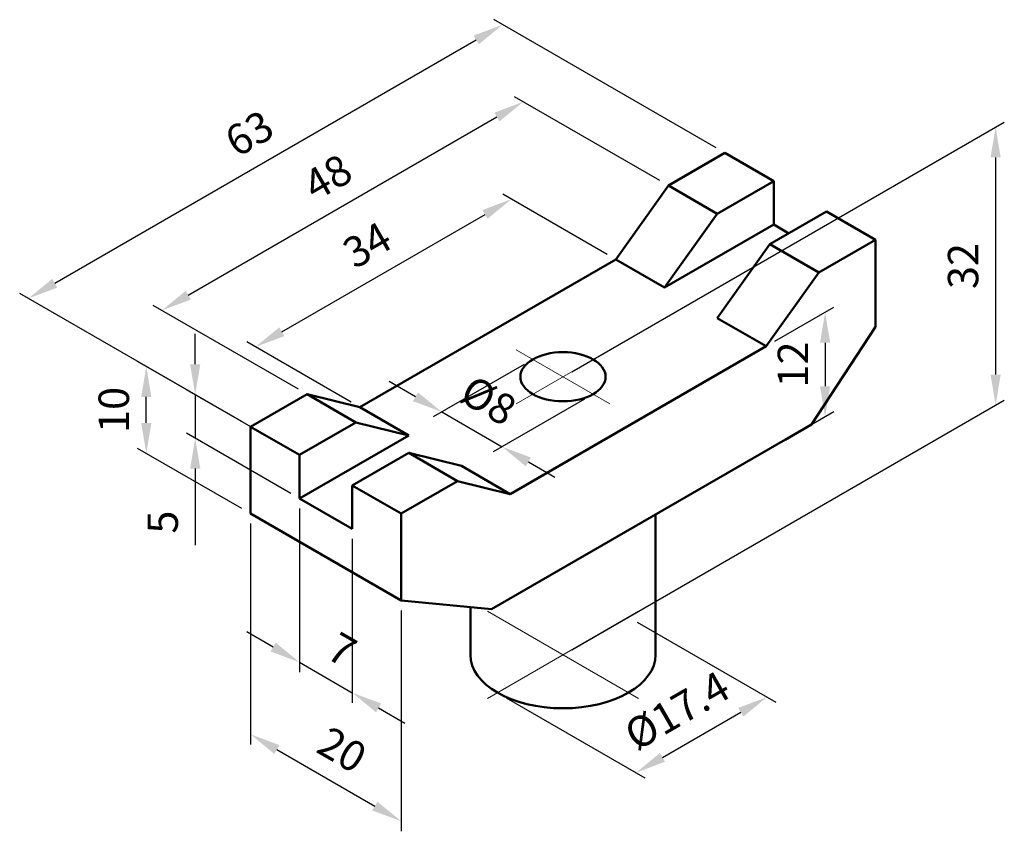
# Model space of a CAD drawing. Units: millimetres. Extents: x 2104 to 2217, y 1234 to 1327.
import ezdxf

# ---------------------------------------------------------------- set-up
doc = ezdxf.new("R2010")
doc.units = ezdxf.units.MM
doc.linetypes.add('CENTER', pattern=[50.8, 31.75, -6.35, 6.35, -6.35])
for name, color, linetype, lineweight in [('M-CNTR', 4, 'CENTER', 18), ('M-DIMS', 3, 'Continuous', 25), ('M-OUTL', 7, 'Continuous', 50)]:
    doc.layers.add(name, color=color, linetype=linetype, lineweight=lineweight)
doc.styles.get("Standard").update_dxf_attribs({"font": 'arial.ttf'})
doc.dimstyles.new('AM_ISO$0', dxfattribs={"dimtxt": 3.5, "dimasz": 3.5, "dimexe": 1, "dimexo": 1, "dimgap": 1.5, "dimtad": 1, "dimdsep": 46, "dimtxsty": 'Standard', "dimcen": 0, "dimclrd": 256, "dimclre": 256, "dimclrt": 2, "dimadec": 0, "dimazin": 2, "dimtp": 0.1, "dimtm": 0.1, "dimtfac": 0.71, "dimtdec": 3, "dimtmove": 0, "dimatfit": 3, "dimfxl": 1, "dimlwd": -1, "dimlwe": -1, "dimarcsym": 1})

# ---------------------------------------------------------------- blocks, each defined once
blk = doc.blocks.new('*D3')
at = {"layer": 'Defpoints', "color": 0, "transparency": 16777216}
for p in [(2159.14, 1326.8), (2184.7, 1312.04), (2130.15, 1280.54)]:
    blk.add_point(p, dxfattribs=at)
at = {"layer": 'M-DIMS', "color": 0, "linetype": 'ByBlock', "transparency": 16777216}
for p, q in [((2183.7, 1312.62), (2158.14, 1327.38)), ((2107.61, 1297.05), (2156.11, 1325.05)), ((2129.15, 1281.12), (2103.58, 1295.88))]:
    blk.add_line(p, q, dxfattribs=at)
at = {"layer": 'M-DIMS', "color": 0, "transparency": 16777216}
for points in [[(2155.82, 1325.55), (2156.4, 1324.54), (2159.14, 1326.8)], [(2107.32, 1297.55), (2107.9, 1296.54), (2104.58, 1295.3)]]:
    blk.add_solid(points, dxfattribs=at)
at = {"layer": 'M-DIMS', "color": 0, "transparency": 16777216, "insert": (2130.22, 1313.9), "char_height": 3.5, "attachment_point": 5, "rotation": 30}
blk.add_mtext('63', dxfattribs=at)
blk = doc.blocks.new('*D4')
at = {"layer": 'Defpoints', "color": 0, "transparency": 16777216}
for p in [(2161.52, 1317.93), (2178.21, 1308.29), (2136.64, 1284.29)]:
    blk.add_point(p, dxfattribs=at)
at = {"layer": 'M-DIMS', "color": 0, "linetype": 'ByBlock', "transparency": 16777216}
for p, q in [((2177.21, 1308.87), (2160.52, 1318.5)), ((2122.98, 1295.68), (2158.49, 1316.18)), ((2135.64, 1284.87), (2118.95, 1294.5))]:
    blk.add_line(p, q, dxfattribs=at)
at = {"layer": 'M-DIMS', "color": 0, "transparency": 16777216}
for points in [[(2158.2, 1316.68), (2158.78, 1315.67), (2161.52, 1317.93)], [(2122.69, 1296.18), (2123.27, 1295.17), (2119.95, 1293.93)]]:
    blk.add_solid(points, dxfattribs=at)
at = {"layer": 'M-DIMS', "color": 0, "transparency": 16777216, "insert": (2139.24, 1308.86), "char_height": 3.5, "attachment_point": 5, "rotation": 30}
blk.add_mtext('48', dxfattribs=at)
blk = doc.blocks.new('*D5')
at = {"layer": 'Defpoints', "color": 0, "transparency": 16777216}
for p in [(2160.15, 1306.72), (2172.15, 1299.79), (2142.7, 1282.79)]:
    blk.add_point(p, dxfattribs=at)
at = {"layer": 'M-DIMS', "color": 0, "linetype": 'ByBlock', "transparency": 16777216}
for p, q in [((2171.15, 1300.37), (2159.15, 1307.3)), ((2133.73, 1291.47), (2157.12, 1304.97)), ((2141.7, 1283.37), (2129.7, 1290.3))]:
    blk.add_line(p, q, dxfattribs=at)
at = {"layer": 'M-DIMS', "color": 0, "transparency": 16777216}
for points in [[(2156.82, 1305.47), (2157.41, 1304.46), (2160.15, 1306.72)], [(2133.44, 1291.97), (2134.03, 1290.96), (2130.7, 1289.72)]]:
    blk.add_solid(points, dxfattribs=at)
at = {"layer": 'M-DIMS', "color": 0, "transparency": 16777216, "insert": (2143.78, 1301.07), "char_height": 3.5, "attachment_point": 5, "rotation": 30}
blk.add_mtext('34', dxfattribs=at)
blk = doc.blocks.new('*D6')
at = {"layer": 'Defpoints', "color": 0, "transparency": 16777216}
for p in [(2118.15, 1287.47), (2130.15, 1280.54), (2130.15, 1270.54)]:
    blk.add_point(p, dxfattribs=at)
at = {"layer": 'M-DIMS', "color": 0, "linetype": 'ByBlock', "transparency": 16777216}
for p, q in [((2129.15, 1281.12), (2117.15, 1288.05)), ((2118.15, 1280.97), (2118.15, 1283.97)), ((2129.15, 1271.12), (2117.15, 1278.05))]:
    blk.add_line(p, q, dxfattribs=at)
at = {"layer": 'M-DIMS', "color": 0, "transparency": 16777216}
for points in [[(2117.56, 1283.97), (2118.73, 1283.97), (2118.15, 1287.47)], [(2117.56, 1280.97), (2118.73, 1280.97), (2118.15, 1277.47)]]:
    blk.add_solid(points, dxfattribs=at)
at = {"layer": 'M-DIMS', "color": 0, "transparency": 16777216, "insert": (2114.86, 1282.47), "char_height": 3.5, "attachment_point": 5, "rotation": 90}
blk.add_mtext('10', dxfattribs=at)
blk = doc.blocks.new('*D7')
at = {"layer": 'Defpoints', "color": 0, "transparency": 16777216}
for p in [(2135.77, 1272.29), (2141.84, 1268.79), (2141.84, 1249.93)]:
    blk.add_point(p, dxfattribs=at)
at = {"layer": 'M-DIMS', "color": 0, "linetype": 'ByBlock', "transparency": 16777216}
for p, q in [((2135.77, 1271.14), (2135.77, 1252.28)), ((2141.84, 1267.64), (2141.84, 1248.78)), ((2132.74, 1255.18), (2129.71, 1256.93)), ((2135.77, 1253.43), (2141.84, 1249.93)), ((2144.87, 1248.18), (2147.9, 1246.43))]:
    blk.add_line(p, q, dxfattribs=at)
at = {"layer": 'M-DIMS', "color": 0, "transparency": 16777216}
for points in [[(2133.03, 1255.69), (2132.45, 1254.68), (2135.77, 1253.43)], [(2145.16, 1248.69), (2144.58, 1247.68), (2141.84, 1249.93)]]:
    blk.add_solid(points, dxfattribs=at)
at = {"layer": 'M-DIMS', "color": 0, "transparency": 16777216, "insert": (2140.43, 1254.5), "char_height": 3.5, "attachment_point": 5, "rotation": 330}
blk.add_mtext('7', dxfattribs=at)
blk = doc.blocks.new('*D8')
at = {"layer": 'Defpoints', "color": 0, "transparency": 16777216}
for p in [(2130.15, 1270.54), (2147.47, 1260.54), (2147.47, 1235.14)]:
    blk.add_point(p, dxfattribs=at)
at = {"layer": 'M-DIMS', "color": 0, "linetype": 'ByBlock', "transparency": 16777216}
for p, q in [((2130.15, 1269.39), (2130.15, 1243.98)), ((2147.47, 1259.39), (2147.47, 1233.98)), ((2133.18, 1243.39), (2144.43, 1236.89))]:
    blk.add_line(p, q, dxfattribs=at)
at = {"layer": 'M-DIMS', "color": 0, "transparency": 16777216}
for points in [[(2133.47, 1243.89), (2132.88, 1242.88), (2130.15, 1245.14)], [(2144.73, 1237.39), (2144.14, 1236.38), (2147.47, 1235.14)]]:
    blk.add_solid(points, dxfattribs=at)
at = {"layer": 'M-DIMS', "color": 0, "transparency": 16777216, "insert": (2140.45, 1242.98), "char_height": 3.5, "attachment_point": 5, "rotation": 330}
blk.add_mtext('20', dxfattribs=at)
blk = doc.blocks.new('*D9')
at = {"layer": 'Defpoints', "color": 0, "transparency": 16777216}
for p in [(2162.62, 1288.29), (2169.55, 1284.29), (2159.07, 1278.24)]:
    blk.add_point(p, dxfattribs=at)
at = {"layer": 'M-DIMS', "color": 0, "linetype": 'ByBlock', "transparency": 16777216}
for p, q in [((2161.62, 1287.71), (2151.14, 1281.66)), ((2149.11, 1283.99), (2146.08, 1285.74)), ((2168.55, 1283.71), (2158.07, 1277.66)), ((2152.14, 1282.24), (2159.07, 1278.24)), ((2162.1, 1276.49), (2165.13, 1274.74))]:
    blk.add_line(p, q, dxfattribs=at)
at = {"layer": 'M-DIMS', "color": 0, "transparency": 16777216}
for points in [[(2149.4, 1284.49), (2148.82, 1283.48), (2152.14, 1282.24)], [(2162.39, 1276.99), (2161.81, 1275.98), (2159.07, 1278.24)]]:
    blk.add_solid(points, dxfattribs=at)
at = {"layer": 'M-DIMS', "color": 0, "transparency": 16777216, "insert": (2157.3, 1283.17), "char_height": 3.5, "attachment_point": 5, "rotation": 330}
blk.add_mtext('%%C8', dxfattribs=at)
blk = doc.blocks.new('*D10')
at = {"layer": 'Defpoints', "color": 0, "transparency": 16777216}
for p in [(2166.09, 1286.29), (2215.86, 1283.03), (2166.09, 1254.29)]:
    blk.add_point(p, dxfattribs=at)
at = {"layer": 'M-DIMS', "color": 0, "linetype": 'ByBlock', "transparency": 16777216}
for p, q in [((2167.09, 1286.87), (2216.86, 1315.6)), ((2215.86, 1311.53), (2215.86, 1286.53)), ((2167.09, 1254.87), (2216.86, 1283.6))]:
    blk.add_line(p, q, dxfattribs=at)
at = {"layer": 'M-DIMS', "color": 0, "transparency": 16777216}
for points in [[(2215.27, 1311.53), (2216.44, 1311.53), (2215.86, 1315.03)], [(2215.27, 1286.53), (2216.44, 1286.53), (2215.86, 1283.03)]]:
    blk.add_solid(points, dxfattribs=at)
at = {"layer": 'M-DIMS', "color": 0, "transparency": 16777216, "insert": (2212.57, 1299.03), "char_height": 3.5, "attachment_point": 5, "rotation": 90}
blk.add_mtext('32', dxfattribs=at)
blk = doc.blocks.new('*D11')
at = {"layer": 'Defpoints', "color": 0, "transparency": 16777216}
for p in [(2189.47, 1289.79), (2196.24, 1281.7), (2189.37, 1277.73)]:
    blk.add_point(p, dxfattribs=at)
at = {"layer": 'M-DIMS', "color": 0, "linetype": 'ByBlock', "transparency": 16777216}
for p, q in [((2190.47, 1290.37), (2197.24, 1294.28)), ((2196.24, 1290.2), (2196.24, 1285.2)), ((2190.37, 1278.31), (2197.24, 1282.28))]:
    blk.add_line(p, q, dxfattribs=at)
at = {"layer": 'M-DIMS', "color": 0, "transparency": 16777216}
for points in [[(2195.66, 1290.2), (2196.83, 1290.2), (2196.24, 1293.7)], [(2195.66, 1285.2), (2196.83, 1285.2), (2196.24, 1281.7)]]:
    blk.add_solid(points, dxfattribs=at)
at = {"layer": 'M-DIMS', "color": 0, "transparency": 16777216, "insert": (2192.99, 1287.7), "char_height": 3.5, "attachment_point": 5, "rotation": 90}
blk.add_mtext('12', dxfattribs=at)
blk = doc.blocks.new('*D12')
at = {"layer": 'Defpoints', "color": 0, "transparency": 16777216}
for p in [(2173.62, 1258.64), (2158.55, 1249.94), (2189.57, 1249.43)]:
    blk.add_point(p, dxfattribs=at)
at = {"layer": 'M-DIMS', "color": 0, "linetype": 'ByBlock', "transparency": 16777216}
for p, q in [((2174.62, 1258.06), (2190.57, 1248.85)), ((2159.55, 1249.36), (2175.5, 1240.15)), ((2177.53, 1242.48), (2186.54, 1247.68))]:
    blk.add_line(p, q, dxfattribs=at)
at = {"layer": 'M-DIMS', "color": 0, "transparency": 16777216}
for points in [[(2186.25, 1248.19), (2186.83, 1247.18), (2189.57, 1249.43)], [(2177.24, 1242.99), (2177.82, 1241.98), (2174.5, 1240.73)]]:
    blk.add_solid(points, dxfattribs=at)
at = {"layer": 'M-DIMS', "color": 0, "transparency": 16777216, "insert": (2179.43, 1247.48), "char_height": 3.5, "attachment_point": 5, "rotation": 30}
blk.add_mtext('%%C17.4', dxfattribs=at)
blk = doc.blocks.new('*D13')
at = {"layer": 'Defpoints', "color": 0, "transparency": 16777216}
for p in [(2123.77, 1279.22), (2135.77, 1277.29), (2135.77, 1272.29)]:
    blk.add_point(p, dxfattribs=at)
at = {"layer": 'M-DIMS', "color": 0, "linetype": 'ByBlock', "transparency": 16777216}
for p, q in [((2123.77, 1287.72), (2123.77, 1291.22)), ((2134.77, 1277.87), (2122.77, 1284.8)), ((2123.77, 1284.22), (2123.77, 1279.22)), ((2134.77, 1272.87), (2122.77, 1279.8)), ((2123.77, 1275.72), (2123.77, 1266.9))]:
    blk.add_line(p, q, dxfattribs=at)
at = {"layer": 'M-DIMS', "color": 0, "transparency": 16777216}
for points in [[(2123.19, 1287.72), (2124.36, 1287.72), (2123.77, 1284.22)], [(2123.19, 1275.72), (2124.36, 1275.72), (2123.77, 1279.22)]]:
    blk.add_solid(points, dxfattribs=at)
at = {"layer": 'M-DIMS', "color": 0, "transparency": 16777216, "insert": (2120.49, 1269.56), "char_height": 3.5, "attachment_point": 5, "rotation": 90}
blk.add_mtext('5', dxfattribs=at)

msp = doc.modelspace()

# ---------------------------------------------------------------- linework, layer by layer
at = {"layer": 'M-CNTR', "ltscale": 25}
for p, q in [((2160.701, 1289.398), (2171.469, 1283.181)), ((2160.701, 1283.181), (2171.469, 1289.398))]:
    msp.add_line(p, q, dxfattribs=at)
at = {"layer": 'M-CNTR'}
for p, q in [((2157.394, 1249.272), (2174.776, 1259.307)), ((2157.394, 1259.307), (2174.776, 1249.272))]:
    msp.add_line(p, q, dxfattribs=at)
at = {"layer": 'M-OUTL'}
for p, q in [((2184.705, 1312.04), (2178.209, 1308.29)), ((2184.705, 1312.04), (2190.334, 1308.79)), ((2183.839, 1305.04), (2190.334, 1308.79)), ((2190.334, 1308.79), (2190.334, 1303.79)), ((2178.209, 1308.29), (2172.147, 1299.79)), ((2183.839, 1305.04), (2178.209, 1308.29)), ((2183.839, 1305.04), (2177.776, 1296.54)), ((2189.901, 1301.54), (2196.396, 1305.29)), ((2196.396, 1305.29), (2202.025, 1302.04)), ((2190.334, 1303.79), (2177.776, 1296.54)), ((2190.334, 1303.79), (2192.066, 1302.79)), ((2189.901, 1301.54), (2183.839, 1293.04)), ((2195.53, 1298.29), (2189.901, 1301.54)), ((2202.025, 1302.04), (2195.53, 1298.29)), ((2202.025, 1302.04), (2195.53, 1298.29)), ((2202.025, 1292.04), (2202.025, 1302.04)), ((2202.025, 1302.04), (2202.025, 1297.04)), ((2202.025, 1302.04), (2202.025, 1292.04)), ((2142.702, 1282.79), (2172.147, 1299.79)), ((2177.776, 1296.54), (2172.147, 1299.79)), ((2195.53, 1298.29), (2189.468, 1289.79)), ((2189.468, 1289.79), (2183.839, 1293.04)), ((2194.664, 1280.79), (2202.025, 1292.04)), ((2189.468, 1289.79), (2160.023, 1272.79)), ((2130.145, 1280.54), (2136.64, 1284.29)), ((2136.64, 1284.29), (2130.145, 1280.54)), ((2136.64, 1284.29), (2142.269, 1281.04)), ((2136.64, 1284.29), (2142.702, 1282.79)), ((2148.332, 1279.54), (2142.702, 1282.79)), ((2130.145, 1270.54), (2130.145, 1280.54)), ((2130.145, 1280.54), (2135.774, 1277.29)), ((2130.145, 1280.54), (2130.145, 1275.54)), ((2135.774, 1277.29), (2142.269, 1281.04)), ((2135.774, 1277.29), (2142.269, 1281.04)), ((2142.269, 1281.04), (2148.332, 1279.54)), ((2157.858, 1259.54), (2194.664, 1280.79)), ((2194.664, 1280.79), (2191.633, 1279.04)), ((2191.633, 1279.04), (2194.664, 1280.79)), ((2148.332, 1279.54), (2135.774, 1272.29)), ((2135.774, 1277.29), (2135.774, 1272.29)), ((2141.836, 1273.79), (2148.332, 1277.54)), ((2148.332, 1277.54), (2154.394, 1276.04)), ((2148.332, 1277.54), (2153.961, 1274.29)), ((2160.023, 1272.79), (2154.394, 1276.04)), ((2141.836, 1268.79), (2141.836, 1273.79)), ((2141.836, 1273.79), (2147.466, 1270.54)), ((2153.961, 1274.29), (2147.466, 1270.54)), ((2153.961, 1274.29), (2160.023, 1272.79)), ((2135.774, 1272.29), (2141.836, 1268.79)), ((2147.466, 1260.54), (2130.145, 1270.54)), ((2147.466, 1270.54), (2147.466, 1260.54)), ((2147.466, 1270.54), (2147.466, 1260.54)), ((2176.74, 1254.29), (2176.74, 1270.442)), ((2147.466, 1260.54), (2157.858, 1259.54)), ((2155.43, 1254.29), (2155.43, 1259.773))]:
    msp.add_line(p, q, dxfattribs=at)
msp.add_ellipse((2166.085, 1286.29), major_axis=(-4.899, 0), ratio=0.5773503, dxfattribs=at)
msp.add_ellipse((2166.085, 1254.29), major_axis=(10.655, 0), ratio=0.5773503, start_param=3.1415927, end_param=6.2831853, dxfattribs=at)

# ---------------------------------------------------------------- dimensions: what is measured, and where the dimension line sits
at = {"layer": 'M-DIMS'}
for p1, p2, distance, override, picture, middle in [((2130.145, 1280.54), (2184.705, 1312.04), 25.563, {"dimpost": '', "dimclrd": 0, "dimclre": 0, "dimclrt": 0}, '*D3', (2130.217, 1313.896)), ((2142.702, 1282.79), (2172.147, 1299.79), 12, {"dimclrd": 0, "dimclre": 0, "dimclrt": 0}, '*D5', (2143.781, 1301.066)), ((2135.774, 1272.29), (2141.836, 1268.79), -16.33, {"dimpost": '', "dimclrd": 0, "dimclre": 0, "dimclrt": 0}, '*D7', (2140.43, 1254.498)), ((2130.145, 1270.54), (2147.466, 1260.54), -22, {"dimclrd": 0, "dimclre": 0, "dimclrt": 0}, '*D8', (2140.449, 1242.983))]:
    dim = msp.add_aligned_dim(p1=p1, p2=p2, distance=distance, dimstyle='AM_ISO$0', override=override, dxfattribs=at)
    dim.commit()
    dim.dimension.update_dxf_attribs({"geometry": picture, "text_midpoint": middle})
dim = msp.add_linear_dim(base=(2161.52, 1317.925), p1=(2136.64, 1284.29), p2=(2178.209, 1308.29), angle=30, dimstyle='AM_ISO$0', override={"dimclrd": 0, "dimclre": 0, "dimclrt": 0}, dxfattribs=at)
dim.commit()
dim.dimension.update_dxf_attribs({"geometry": '*D4', "text_midpoint": (2140.887, 1306.013), "dimtype": 161})
for base, p1, p2, override, picture, middle in [((2215.857, 1283.026), (2166.085, 1286.29), (2166.085, 1254.29), {"dimpost": '', "dimclrd": 0, "dimclre": 0, "dimclrt": 0}, '*D10', (2212.569, 1299.026)), ((2123.774, 1279.218), (2135.774, 1277.29), (2135.774, 1272.29), {"dimpost": '', "dimclrd": 0, "dimclre": 0, "dimclrt": 0}, '*D13', (2120.494, 1269.558)), ((2118.145, 1287.468), (2130.145, 1270.54), (2130.145, 1280.54), {"dimclrd": 0, "dimclre": 0, "dimclrt": 0}, '*D6', (2114.858, 1282.468))]:
    dim = msp.add_linear_dim(base=base, p1=p1, p2=p2, angle=90, dimstyle='AM_ISO$0', override=override, dxfattribs=at)
    dim.commit()
    dim.dimension.update_dxf_attribs({"geometry": picture, "text_midpoint": middle})
dim = msp.add_linear_dim(base=(2196.244, 1281.702), p1=(2189.468, 1289.79), p2=(2189.365, 1277.731), angle=90, text='12', dimstyle='AM_ISO$0', override={"dimpost": '', "dimclrd": 0, "dimclre": 0, "dimclrt": 0}, dxfattribs=at)
dim.commit()
dim.dimension.update_dxf_attribs({"geometry": '*D11', "text_midpoint": (2192.987, 1287.702)})
for base, p1, p2, angle, picture, middle in [((2159.067, 1278.238), (2162.621, 1288.29), (2169.549, 1284.29), 330, '*D9', (2155.603, 1280.238)), ((2189.57, 1249.43), (2158.551, 1249.94), (2173.619, 1258.64), 30, '*D12', (2181.122, 1244.553))]:
    dim = msp.add_linear_dim(base=base, p1=p1, p2=p2, angle=angle, text='%%C<>', dimstyle='AM_ISO$0', override={"dimclrd": 0, "dimclre": 0, "dimclrt": 0}, dxfattribs=at)
    dim.commit()
    dim.dimension.update_dxf_attribs({"geometry": picture, "text_midpoint": middle, "dimtype": 161})

doc.saveas('drawing.dxf')
